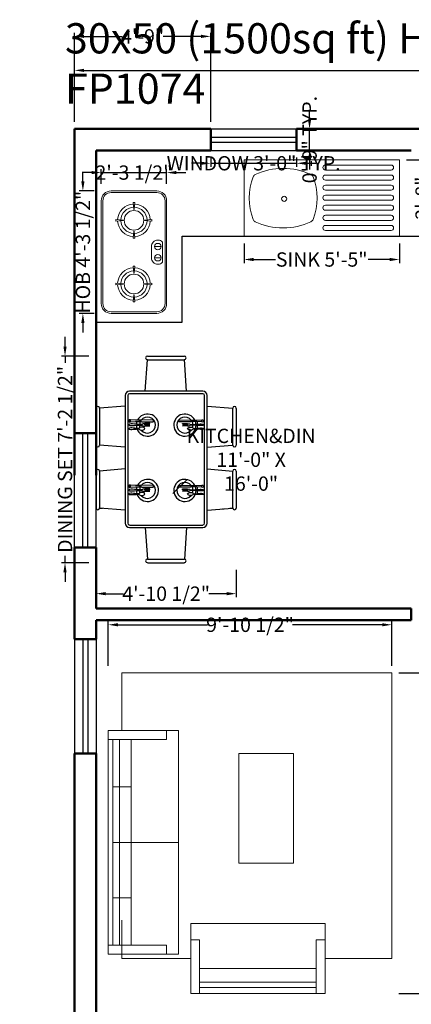
# Model space of a CAD drawing. Units: inches. Extents: x 234 to 707, y 260 to 1025.
# Tile 2 of 3: x 234 to 398, y 612 to 1025. Entities that reach past the tile are written whole.
import ezdxf

# ---------------------------------------------------------------- set-up
doc = ezdxf.new("R2010")
doc.units = ezdxf.units.IN
doc.header["$MEASUREMENT"] = 0
doc.layers.add('a patt', color=33, linetype='Continuous')
for name, color, linetype, lineweight in [('A-ANNO-DIMS', 3, 'Continuous', 18), ('A-ANNO-TEXT', 7, 'Continuous', 35), ('A-AREA-IDEN', 7, 'Continuous', 25), ('A-EQPM', 8, 'Continuous', 18), ('A-FLOR-CASE', 30, 'Continuous', 25), ('A-FLOR-FIXT', 9, 'Continuous', 18), ('A-FURN', 9, 'Continuous', 18), ('WALL', 7, 'Continuous', 50), ('WINDOW', 2, 'Continuous', 25)]:
    doc.layers.add(name, color=color, linetype=linetype, lineweight=lineweight)
doc.styles.get("Standard").update_dxf_attribs({"font": 'arial.ttf'})
doc.styles.add('YQ_DIM', font='SUPEROS.SHX', dxfattribs={"width": 0.8, "bigfont": 'HZDX.SHX'})
doc.dimstyles.new('yqi0', dxfattribs={"dimscale": 0, "dimtxt": 6, "dimasz": 4, "dimexe": 1.5, "dimexo": 3, "dimgap": 0.5, "dimtad": 0, "dimdec": 1, "dimdsep": 46, "dimlunit": 4, "dimtxsty": 'Standard', "dimcen": 0, "dimclrd": 256, "dimclre": 256, "dimclrt": 7, "dimadec": 1, "dimazin": 2, "dimtfac": 1, "dimtdec": 1, "dimtix": 1, "dimtmove": 2, "dimatfit": 2, "dimfxl": 1, "dimtolj": 1, "dimtzin": 0, "dimarcsym": 0})

# ---------------------------------------------------------------- blocks, each defined once
blk = doc.blocks.new('*D2')
at = {"layer": 'A-ANNO-DIMS', "color": 0, "lineweight": -2, "transparency": 16777216}
for p, q in [((257.21, 981.74), (257.21, 1004.79)), ((261.21, 1003.29), (431.62, 1003.29)), ((613.21, 1003.29), (442.8, 1003.29)), ((617.21, 981.74), (617.21, 1004.79))]:
    blk.add_line(p, q, dxfattribs=at)
at = {"layer": 'A-ANNO-DIMS', "color": 0, "transparency": 16777216}
for points in [[(261.21, 1003.95), (261.21, 1002.62), (257.21, 1003.29)], [(613.21, 1003.95), (613.21, 1002.62), (617.21, 1003.29)]]:
    blk.add_solid(points, dxfattribs=at)
at = {"layer": 'Defpoints', "color": 0, "transparency": 16777216}
for p in [(617.21, 1003.29), (257.21, 978.74), (617.21, 978.74)]:
    blk.add_point(p, dxfattribs=at)
at = {"layer": 'A-ANNO-DIMS', "color": 0, "transparency": 16777216, "insert": (437.21, 1003.29), "char_height": 6, "attachment_point": 5}
blk.add_mtext("\\A1;30'", dxfattribs=at)
blk = doc.blocks.new('WD_WIN4')
for p, q in [((-0.5, 0.5), (0.5, 0.5)), ((-0.5, 0.12), (0.5, 0.12)), ((-0.5, -0.12), (0.5, -0.12)), ((-0.5, -0.5), (0.5, -0.5))]:
    blk.add_line(p, q)
blk = doc.blocks.new('yq_cooker_01')
for p, q in [((426.3, 34.3), (465.5, 34.3)), ((426.3, -34.3), (465.5, -34.3))]:
    blk.add_line(p, q)
for points in [[(440, -375), (160, -375, -0.414214), (100, -315), (100, 315, -0.414214), (160, 375), (440, 375, -0.414214), (500, 315), (500, -315, -0.414214)], [(440, -365), (160, -365, -0.414214), (110, -315), (110, 315, -0.414214), (160, 365), (440, 365, -0.414214), (490, 315), (490, -315, -0.414214)]]:
    blk.add_lwpolyline(points, format="xyb", close=True)
for points in [[(300.8, 261.3), (305.4, 305), (294.6, 305), (299.2, 261.3)], [(233.7, 195.8), (190, 200.4), (190, 189.6), (233.7, 194.2)], [(366.3, 194.2), (410, 189.6), (410, 200.4), (366.3, 195.8)], [(299.2, 128.7), (294.6, 85), (305.4, 85), (300.8, 128.7)], [(299.2, -128.7), (294.6, -85), (305.4, -85), (300.8, -128.7)], [(233.7, -195.8), (190, -200.4), (190, -189.6), (233.7, -194.2)], [(366.3, -194.2), (410, -189.6), (410, -200.4), (366.3, -195.8)], [(300.8, -261.3), (305.4, -305), (294.6, -305), (299.2, -261.3)]]:
    blk.add_lwpolyline(points, close=True)
blk.add_lwpolyline([(406.7, -34.3, 0.414214), (445.9, -73.5), (455.5, -73.5, 0.414214), (475.1, -53.9), (475.1, 53.9, 0.414214), (455.5, 73.5), (445.9, 73.5, 0.414214), (406.7, 34.3), (406.7, -34.3)], format="xyb")
for centre, radius in [((300, 195), 60), ((445.9, 34.3), 19.6), ((445.9, -34.3), 19.6), ((300, -195), 60)]:
    blk.add_circle(centre, radius)
for centre, radius, start, end in [((300, 195), 100, 92.4978, 177.5022), ((300, 195), 80, 91.59131, 178.40869), ((300, 195), 80, 1.59131, 88.40869), ((300, 195), 100, 2.4978, 87.5022), ((300, 195), 100, 182.4978, 267.5022), ((300, 195), 80, 181.59131, 268.40869), ((300, 195), 80, 271.59131, 358.40869), ((300, 195), 100, 272.4978, 357.5022), ((300, -195), 100, 92.4978, 177.5022), ((300, -195), 80, 91.59131, 178.40869), ((300, -195), 80, 1.59131, 88.40869), ((300, -195), 100, 2.4978, 87.5022), ((300, -195), 100, 182.4978, 267.5022), ((300, -195), 80, 181.59131, 268.40869), ((300, -195), 80, 271.59131, 358.40869), ((300, -195), 100, 272.4978, 357.5022)]:
    blk.add_arc(centre, radius, start, end)
blk = doc.blocks.new('sink7a')
for p, q in [((12297, -765), (22250, -765)), ((12297, -1527), (22250, -1527)), ((12297, -2289), (22250, -2289)), ((12297, -3051), (22250, -3051)), ((12297, -3813), (22250, -3813)), ((12297, -4575), (22250, -4575)), ((12297, -5337), (22250, -5337)), ((12297, -6099), (22250, -6099)), ((12297, -6861), (22250, -6861)), ((12297, -7623), (22250, -7623)), ((12297, -8385), (22250, -8385)), ((12297, -9147), (22250, -9147)), ((12297, -9909), (22250, -9909)), ((12297, -10671), (22250, -10671))]:
    blk.add_line(p, q)
blk.add_lwpolyline([(0, 0), (0, -11557), (23495, -11557), (23495, 0)], close=True)
blk.add_lwpolyline([(1692, -9356, -0.193356), (1368, -9011, -0.1886606), (1376, -2541, -0.1929606), (1700, -2197, -0.2205414), (10111, -2197, -0.1929606), (10435, -2541, -0.1886606), (10443, -9011, -0.193356), (10119, -9356, -0.2209789)], format="xyb", close=True)
blk.add_circle((6064, -5888), 381)
for centre, start, end in [((12297, -1146), 90, 270), ((22250, -1146), 270, 90), ((12297, -2670), 90, 270), ((22250, -2670), 270, 90), ((12297, -4194), 90, 270), ((22250, -4194), 270, 90), ((12297, -5718), 90, 270), ((22250, -5718), 270, 90), ((12297, -7242), 90, 270), ((22250, -7242), 270, 90), ((12297, -8766), 90, 270), ((22250, -8766), 270, 90), ((12297, -10290), 90, 270), ((22250, -10290), 270, 90)]:
    blk.add_arc(centre, 381, start, end)
blk = doc.blocks.new('SOFA 21')
for p, q in [((-49.09, -24.34), (-49.09, 0)), ((37.16, -24.34), (37.16, 0)), ((-29.27, -1.86), (-49.09, -1.86)), ((-29.27, -9.53), (-29.27, -1.86)), ((-29.27, -1.86), (-5.97, -1.86)), ((17.33, -1.86), (-5.97, -1.86)), ((-5.97, -1.86), (-5.97, -9.53)), ((17.33, -9.53), (17.33, -1.86)), ((17.33, -1.86), (37.16, -1.86)), ((37.16, -4.72), (-49.09, -4.72)), ((37.16, -9.53), (-49.09, -9.53)), ((-5.97, -9.53), (-5.97, -29.38)), ((-52.84, -24.34), (-49.09, -24.34)), ((40.91, -24.34), (37.16, -24.34)), ((-46.78, -38.24), (-46.78, -34.49)), ((-46.78, -38.24), (-69.34, -38.24)), ((-66.74, -38.24), (-66.74, -86.99)), ((-64.62, -86.99), (-64.62, -38.24)), ((-58.88, -38.24), (-58.88, -86.99)), ((-46.78, -86.99), (-69.34, -86.99)), ((-46.78, -86.99), (-46.78, -90.74))]:
    blk.add_line(p, q)
for points in [[(40.91, -29.38), (-52.84, -29.38), (-52.84, 0), (40.91, 0)], [(-69.34, -34.49), (-69.34, -90.74), (-39.97, -90.74), (-39.97, -34.49)]]:
    blk.add_lwpolyline(points, close=True)
at = {"color": 0, "linetype": 'ByBlock', "lineweight": -2}
for points in [[(-54.65, -34.49), (-54.65, -5.62)], [(-54.65, -5.62), (-38.57, -5.62)], [(40.91, -5.62), (65.11, -5.62), (65.11, -118.7), (34.12, -118.7)], [(34.12, -118.7), (-54.65, -118.7), (-54.65, -90.74)]]:
    blk.add_lwpolyline(points, dxfattribs=at)
blk.add_lwpolyline([(-14.65, -77.55), (31.25, -77.55), (31.25, -54.6), (-14.65, -54.6)], close=True, dxfattribs=at)
blk = doc.blocks.new('grdfg')
at = {"layer": 'a patt'}
for p, q in [((589, 1028), (612, 1310)), ((609, 1310), (609, 1278)), ((615, 1349), (612, 1349)), ((1019, 1310), (612, 1310)), ((1016, 1349), (615, 1349)), ((615, 1349), (615, 1349)), ((1016, 1349), (1019, 1349)), ((1042, 1028), (1019, 1310)), ((1281, 1028), (1304, 1310)), ((1307, 1349), (1304, 1349)), ((1711, 1310), (1304, 1310)), ((1307, 1349), (1307, 1349)), ((1708, 1349), (1307, 1349)), ((1708, 1349), (1711, 1349)), ((1734, 1028), (1711, 1310)), ((605, 1201), (603, 1201)), ((1297, 1201), (1295, 1201)), ((397, 982), (397, 175)), ((425, 982), (425, 175)), ((1851, 1028), (444, 1028)), ((1851, 1000), (444, 1000)), ((1869, 175), (1869, 982)), ((1897, 175), (1897, 982)), ((763, 888), (769, 888)), ((763, 879), (769, 879)), ((841, 970), (863, 970)), ((845, 870), (859, 870)), ((1482, 888), (1488, 888)), ((1482, 879), (1488, 879)), ((1560, 970), (1582, 970)), ((1564, 870), (1578, 870)), ((10, 785), (10, 378)), ((397, 808), (49, 782)), ((49, 782), (49, 785)), ((49, 782), (49, 381)), ((813, 857), (806, 857)), ((806, 845), (813, 845)), ((845, 859), (859, 859)), ((845, 852), (859, 852)), ((1532, 857), (1525, 857)), ((1525, 845), (1532, 845)), ((1564, 859), (1578, 859)), ((1564, 852), (1578, 852)), ((1897, 808), (2245, 782)), ((2245, 782), (2246, 785)), ((2245, 782), (2245, 381)), ((2285, 785), (2285, 378)), ((770, 505), (923, 352)), ((49, 381), (49, 378)), ((49, 381), (49, 381)), ((397, 355), (49, 375)), ((1897, 355), (2246, 375)), ((2246, 381), (2245, 381)), ((2245, 381), (2246, 378)), ((763, 277), (769, 277)), ((763, 268), (769, 268)), ((771, 235), (802, 235)), ((806, 312), (813, 312)), ((813, 299), (806, 299)), ((816, 235), (844, 235)), ((845, 305), (859, 305)), ((845, 297), (859, 297)), ((845, 287), (859, 287)), ((1482, 277), (1488, 277)), ((1482, 268), (1488, 268)), ((1490, 235), (1521, 235)), ((1525, 312), (1532, 312)), ((1532, 299), (1525, 299)), ((1535, 235), (1563, 235)), ((1564, 305), (1578, 305)), ((1564, 297), (1578, 297)), ((1564, 287), (1578, 287)), ((444, 156), (1851, 156)), ((444, 128), (1851, 128)), ((589, 128), (612, -153)), ((841, 187), (863, 187)), ((1042, 128), (1019, -154)), ((1281, 128), (1304, -153)), ((1560, 187), (1582, 187)), ((1734, 128), (1711, -154)), ((605, -45), (603, -45)), ((1028, -45), (1026, -45)), ((609, -122), (609, -154)), ((1019, -153), (612, -153)), ((615, -193), (612, -193)), ((615, -192), (615, -193)), ((1016, -193), (615, -193)), ((1016, -193), (1019, -193)), ((1711, -153), (1304, -153)), ((1307, -193), (1304, -193)), ((1307, -192), (1307, -193)), ((1708, -193), (1307, -193)), ((1708, -193), (1711, -193))]:
    blk.add_line(p, q, dxfattribs=at)
for points in [[(759, 967), (759, 955, -0.013852), (763, 888), (763, 879, -0.321801), (758, 871, 0.220637), (749, 856, 0.151079), (756, 820, 0.601255), (777, 820, 0.098298), (784, 846, 0.173345), (779, 867, 0.127575), (772, 873, -0.108886), (769, 879), (769, 888, -0.013852), (774, 955), (774, 967), (772, 982, 0.903848), (760, 982)], [(841, 986, 0.204141), (841, 970), (845, 914), (845, 870), (843, 863), (845, 859), (845, 852), (843, 847, -0.015744), (841, 722, 0.538165), (859, 722), (864, 847), (859, 852), (859, 859), (861, 863), (859, 870), (859, 914), (863, 970, 0.204141), (863, 986), (857, 988), (847, 988)], [(1478, 967), (1478, 955, -0.013852), (1482, 888), (1482, 879, -0.321801), (1477, 871, 0.220637), (1468, 856, 0.151079), (1475, 820, 0.601255), (1496, 820, 0.098298), (1503, 846, 0.173345), (1498, 867, 0.127575), (1491, 873, -0.108886), (1488, 879), (1488, 888, -0.013852), (1493, 955), (1493, 967), (1491, 982, 0.903848), (1479, 982)], [(1560, 986, 0.204141), (1560, 970), (1564, 914), (1564, 870), (1562, 863), (1564, 859), (1564, 852), (1562, 847, -0.015744), (1560, 722, 0.538165), (1578, 722), (1583, 847), (1578, 852), (1578, 859), (1580, 863), (1578, 870), (1578, 914), (1582, 970, 0.204141), (1582, 986), (1576, 988), (1566, 988)], [(841, 171, -0.204141), (841, 187), (845, 242), (845, 287), (843, 294), (845, 297), (845, 305), (843, 310, 0.015744), (841, 435, -0.538165), (859, 435), (864, 310), (859, 305), (859, 297), (861, 294), (859, 287), (859, 242), (863, 187, -0.204141), (863, 171), (857, 169), (847, 169)], [(1560, 171, -0.204141), (1560, 187), (1564, 242), (1564, 287), (1562, 294), (1564, 297), (1564, 305), (1562, 310, 0.015744), (1560, 435, -0.538165), (1578, 435), (1583, 310), (1578, 305), (1578, 297), (1580, 294), (1578, 287), (1578, 242), (1582, 187, -0.204141), (1582, 171), (1576, 169), (1566, 169)], [(759, 189), (759, 202, 0.013852), (763, 268), (763, 277, 0.321801), (758, 285, -0.220637), (749, 300, -0.151079), (756, 336, -0.601255), (777, 336, -0.098298), (784, 311, -0.173345), (779, 289, -0.127575), (772, 283, 0.108886), (769, 277), (769, 268, 0.013852), (774, 202), (774, 189), (772, 174, -0.903848), (760, 174)], [(1478, 189), (1478, 202, 0.013852), (1482, 268), (1482, 277, 0.321801), (1477, 285, -0.220637), (1468, 300, -0.151079), (1475, 336, -0.601255), (1496, 336, -0.098298), (1503, 311, -0.173345), (1498, 289, -0.127575), (1491, 283, 0.108886), (1488, 277), (1488, 268, 0.013852), (1493, 202), (1493, 189), (1491, 174, -0.903848), (1479, 174)]]:
    blk.add_lwpolyline(points, format="xyb", close=True, dxfattribs=at)
for points in [[(802, 982), (800, 964), (800, 950, -0.012883), (806, 857), (806, 845, -0.236068), (798, 834, 0.098033), (795, 814), (797, 759), (798, 759), (800, 814), (802, 814), (804, 759), (806, 759), (807, 816), (809, 818), (811, 816), (813, 759), (814, 759), (816, 814), (818, 814), (820, 759), (822, 759), (823, 814), (820, 834, -0.236068), (813, 845), (813, 857, -0.012883), (818, 950), (818, 964), (816, 982, 0.761905), (802, 982, 0.027392)], [(1521, 982), (1519, 964), (1519, 950, -0.012883), (1525, 857), (1525, 845, -0.236068), (1517, 834, 0.098033), (1514, 814), (1516, 759), (1517, 759), (1519, 814), (1521, 814), (1523, 759), (1525, 759), (1526, 816), (1528, 818), (1530, 816), (1532, 759), (1533, 759), (1535, 814), (1537, 814), (1539, 759), (1541, 759), (1542, 814), (1539, 834, -0.236068), (1532, 845), (1532, 857, -0.012883), (1537, 950), (1537, 964), (1535, 982, 0.761905), (1521, 982, 0.027392)], [(802, 174), (800, 192), (800, 206, 0.012883), (806, 299), (806, 312, 0.236068), (798, 322, -0.098033), (795, 342), (797, 397), (798, 397), (800, 342), (802, 342), (804, 397), (806, 397), (807, 340), (809, 338), (811, 340), (813, 397), (814, 397), (816, 342), (818, 342), (820, 397), (822, 397), (823, 342), (820, 322, 0.236068), (813, 312), (813, 299, 0.012883), (818, 206), (818, 192), (816, 174, -0.761905), (802, 174, -0.027392)], [(1521, 174), (1519, 192), (1519, 206, 0.012883), (1525, 299), (1525, 312, 0.236068), (1517, 322, -0.098033), (1514, 342), (1516, 397), (1517, 397), (1519, 342), (1521, 342), (1523, 397), (1525, 397), (1526, 340), (1528, 338), (1530, 340), (1532, 397), (1533, 397), (1535, 342), (1537, 342), (1539, 397), (1541, 397), (1542, 342), (1539, 322, 0.236068), (1532, 312), (1532, 299, 0.012883), (1537, 206), (1537, 192), (1535, 174, -0.761905), (1521, 174, -0.027392)]]:
    blk.add_lwpolyline(points, format="xyb", dxfattribs=at)
for centre, radius, start, end in [((613, 1329), 19.5, 92.4912, 267.9051), ((1018, 1329), 19.5, 272.0949, 87.5088), ((1305, 1329), 19.5, 92.4912, 267.9051), ((1710, 1329), 19.5, 272.0949, 87.5088), ((444, 982), 46.6, 90, 180), ((444, 982), 18.7, 90, 180), ((1851, 982), 46.6, 0, 90), ((1851, 982), 18.7, 0, 90), ((806, 784), 122, 110.569, 64.0676), ((806, 784), 122, 91.1026, 107.1168), ((806, 784), 88.4, 90.4281, 108.0635), ((806, 784), 88.4, 64.8376, 85.191), ((806, 784), 122, 71.3681, 85.7295), ((1525, 784), 122, 110.569, 64.0676), ((1525, 784), 122, 91.1026, 107.1168), ((1525, 784), 88.4, 90.4281, 108.0635), ((1525, 784), 88.4, 64.8376, 85.191), ((1525, 784), 122, 71.3681, 85.7295), ((30, 784), 19.5, 2.4912, 177.9051), ((806, 784), 88.4, 130.4177, 52.8326), ((1525, 784), 88.4, 130.4177, 52.8326), ((2265, 784), 19.5, 2.0949, 177.5088), ((806, 372), 122, 295.9324, 249.431), ((806, 372), 88.4, 307.1674, 229.5823), ((1525, 372), 122, 295.9324, 249.431), ((1525, 372), 88.4, 307.1674, 229.5823), ((30, 379), 19.5, 182.0949, 357.5088), ((2265, 379), 19.5, 182.4912, 357.9051), ((806, 372), 122, 252.8832, 268.8974), ((806, 372), 88.4, 251.9365, 269.5719), ((806, 372), 88.4, 274.809, 295.1624), ((806, 372), 122, 274.2705, 288.6319), ((1525, 372), 122, 252.8832, 268.8974), ((1525, 372), 88.4, 251.9365, 269.5719), ((1525, 372), 88.4, 274.809, 295.1624), ((1525, 372), 122, 274.2705, 288.6319), ((444, 175), 46.6, 180, 270), ((444, 175), 18.7, 180, 270), ((1851, 175), 46.6, 270, 0), ((1851, 175), 18.7, 270, 0), ((613, -173), 19.5, 92.0949, 267.5088), ((1018, -173), 19.5, 272.4912, 87.9051), ((1305, -173), 19.5, 92.0949, 267.5088), ((1710, -173), 19.5, 272.4912, 87.9051)]:
    blk.add_arc(centre, radius, start, end, dxfattribs=at)
blk = doc.blocks.new('*D23')
at = {"layer": 'A-ANNO-DIMS', "lineweight": -2, "transparency": 16777216}
for p, q in [((314.21, 966.74), (314.21, 962.84)), ((350.21, 966.74), (350.21, 962.84)), ((310.21, 964.34), (306.21, 964.34)), ((314.21, 964.34), (350.21, 964.34)), ((354.21, 964.34), (358.21, 964.34))]:
    blk.add_line(p, q, dxfattribs=at)
at = {"layer": 'A-ANNO-DIMS', "transparency": 16777216}
for points in [[(310.21, 965.01), (310.21, 963.67), (314.21, 964.34)], [(354.21, 965.01), (354.21, 963.67), (350.21, 964.34)]]:
    blk.add_solid(points, dxfattribs=at)
at = {"layer": 'Defpoints', "color": 0, "transparency": 16777216}
for p in [(314.21, 969.74), (350.21, 969.74), (350.21, 964.34)]:
    blk.add_point(p, dxfattribs=at)
at = {"layer": 'A-ANNO-DIMS', "color": 7, "transparency": 16777216, "insert": (332.21, 964.34), "char_height": 6, "attachment_point": 5}
blk.add_mtext('\\A1;WINDOW 3\'-0" TYP.', dxfattribs=at)
blk = doc.blocks.new('*D24')
at = {"layer": 'A-ANNO-DIMS', "lineweight": -2, "transparency": 16777216}
for p, q in [((355.61, 982.74), (355.61, 986.74)), ((353.21, 978.74), (357.11, 978.74)), ((355.61, 969.74), (355.61, 978.74)), ((353.21, 969.74), (357.11, 969.74)), ((355.61, 965.74), (355.61, 961.74))]:
    blk.add_line(p, q, dxfattribs=at)
at = {"layer": 'A-ANNO-DIMS', "transparency": 16777216}
for points in [[(354.95, 982.74), (356.28, 982.74), (355.61, 978.74)], [(354.95, 965.74), (356.28, 965.74), (355.61, 969.74)]]:
    blk.add_solid(points, dxfattribs=at)
at = {"layer": 'Defpoints', "color": 0, "transparency": 16777216}
for p in [(350.21, 978.74), (355.61, 978.74), (350.21, 969.74)]:
    blk.add_point(p, dxfattribs=at)
at = {"layer": 'A-ANNO-DIMS', "color": 7, "transparency": 16777216, "insert": (355.61, 974.24), "char_height": 6, "attachment_point": 5, "rotation": 90}
blk.add_mtext('\\A1;0\'-9" TYP.', dxfattribs=at)
blk = doc.blocks.new('*D39')
at = {"layer": 'A-ANNO-DIMS', "lineweight": -2, "transparency": 16777216}
for p, q in [((260.71, 956.73), (260.71, 960.73)), ((265.41, 952.73), (259.21, 952.73)), ((260.71, 952.73), (260.71, 952.62)), ((265.41, 901.4), (259.21, 901.4)), ((260.71, 901.4), (260.71, 901.52)), ((260.71, 897.4), (260.71, 893.4))]:
    blk.add_line(p, q, dxfattribs=at)
at = {"layer": 'A-ANNO-DIMS', "transparency": 16777216}
for points in [[(260.04, 956.73), (261.37, 956.73), (260.71, 952.73)], [(260.04, 897.4), (261.37, 897.4), (260.71, 901.4)]]:
    blk.add_solid(points, dxfattribs=at)
at = {"layer": 'Defpoints', "color": 0, "transparency": 16777216}
for p in [(260.71, 952.73), (268.41, 952.73), (268.41, 901.4)]:
    blk.add_point(p, dxfattribs=at)
at = {"layer": 'A-ANNO-DIMS', "color": 7, "transparency": 16777216, "insert": (260.71, 927.07), "char_height": 6, "attachment_point": 5, "rotation": 90}
blk.add_mtext('\\A1;HOB 4\'-3 1/2"', dxfattribs=at)
blk = doc.blocks.new('*D40')
at = {"layer": 'A-ANNO-DIMS', "lineweight": -2, "transparency": 16777216}
for p, q in [((268.41, 955.73), (268.41, 961.93)), ((295.78, 955.73), (295.78, 961.93)), ((264.41, 960.43), (260.41, 960.43)), ((268.41, 960.43), (295.78, 960.43)), ((299.78, 960.43), (303.78, 960.43))]:
    blk.add_line(p, q, dxfattribs=at)
at = {"layer": 'A-ANNO-DIMS', "transparency": 16777216}
for points in [[(264.41, 961.1), (264.41, 959.77), (268.41, 960.43)], [(299.78, 961.1), (299.78, 959.77), (295.78, 960.43)]]:
    blk.add_solid(points, dxfattribs=at)
at = {"layer": 'Defpoints', "color": 0, "transparency": 16777216}
for p in [(295.78, 960.43), (268.41, 952.73), (295.78, 952.73)]:
    blk.add_point(p, dxfattribs=at)
at = {"layer": 'A-ANNO-DIMS', "color": 7, "transparency": 16777216, "insert": (282.09, 960.43), "char_height": 6, "attachment_point": 5}
blk.add_mtext('\\A1;2\'-3 1/2"', dxfattribs=at)
blk = doc.blocks.new('*D41')
at = {"layer": 'A-ANNO-DIMS', "lineweight": -2, "transparency": 16777216}
for p, q in [((328.2, 930.74), (328.2, 922.49)), ((393.21, 930.74), (393.21, 922.49)), ((332.2, 923.99), (341.3, 923.99)), ((389.21, 923.99), (380.11, 923.99))]:
    blk.add_line(p, q, dxfattribs=at)
at = {"layer": 'A-ANNO-DIMS', "transparency": 16777216}
for points in [[(332.2, 924.66), (332.2, 923.32), (328.2, 923.99)], [(389.21, 924.66), (389.21, 923.32), (393.21, 923.99)]]:
    blk.add_solid(points, dxfattribs=at)
at = {"layer": 'Defpoints', "color": 0, "transparency": 16777216}
for p in [(328.2, 933.74), (393.21, 933.74), (393.21, 923.99)]:
    blk.add_point(p, dxfattribs=at)
at = {"layer": 'A-ANNO-DIMS', "color": 7, "transparency": 16777216, "insert": (360.7, 923.99), "char_height": 6, "attachment_point": 5}
blk.add_mtext('\\A1;SINK 5\'-5"', dxfattribs=at)
blk = doc.blocks.new('*D42')
at = {"layer": 'A-ANNO-DIMS', "lineweight": -2, "transparency": 16777216}
for p, q in [((396.21, 965.72), (404.46, 965.72)), ((402.96, 961.72), (402.96, 958.26)), ((402.96, 937.74), (402.96, 941.21)), ((396.21, 933.74), (404.46, 933.74))]:
    blk.add_line(p, q, dxfattribs=at)
at = {"layer": 'A-ANNO-DIMS', "transparency": 16777216}
for points in [[(402.3, 961.72), (403.63, 961.72), (402.96, 965.72)], [(402.3, 937.74), (403.63, 937.74), (402.96, 933.74)]]:
    blk.add_solid(points, dxfattribs=at)
at = {"layer": 'Defpoints', "color": 0, "transparency": 16777216}
for p in [(393.21, 965.72), (402.96, 965.72), (393.21, 933.74)]:
    blk.add_point(p, dxfattribs=at)
at = {"layer": 'A-ANNO-DIMS', "color": 7, "transparency": 16777216, "insert": (402.96, 949.73), "char_height": 6, "attachment_point": 5, "rotation": 90}
blk.add_mtext('\\A1;2\'-8"', dxfattribs=at)
blk = doc.blocks.new('*D45')
at = {"layer": 'A-ANNO-DIMS', "lineweight": -2, "transparency": 16777216}
for p, q in [((393.05, 750.69), (411.72, 750.69)), ((410.22, 746.69), (410.22, 729.31)), ((410.22, 620.24), (410.22, 637.63)), ((393.05, 616.24), (411.72, 616.24))]:
    blk.add_line(p, q, dxfattribs=at)
at = {"layer": 'A-ANNO-DIMS', "transparency": 16777216}
for points in [[(409.55, 746.69), (410.88, 746.69), (410.22, 750.69)], [(409.55, 620.24), (410.88, 620.24), (410.22, 616.24)]]:
    blk.add_solid(points, dxfattribs=at)
at = {"layer": 'Defpoints', "color": 0, "transparency": 16777216}
for p in [(390.05, 750.69), (410.22, 750.69), (390.05, 616.24)]:
    blk.add_point(p, dxfattribs=at)
at = {"layer": 'A-ANNO-DIMS', "color": 7, "transparency": 16777216, "insert": (410.22, 683.47), "char_height": 6, "attachment_point": 5, "rotation": 90}
blk.add_mtext('\\A1;LOUNGE SET 11\'-2 1/2"', dxfattribs=at)
blk = doc.blocks.new('*D46')
at = {"layer": 'A-ANNO-DIMS', "lineweight": -2, "transparency": 16777216}
for p, q in [((271.35, 753.69), (271.35, 772.36)), ((390.05, 753.69), (390.05, 772.36)), ((275.35, 770.86), (312.9, 770.86)), ((386.05, 770.86), (348.49, 770.86))]:
    blk.add_line(p, q, dxfattribs=at)
at = {"layer": 'A-ANNO-DIMS', "transparency": 16777216}
for points in [[(275.35, 771.52), (275.35, 770.19), (271.35, 770.86)], [(386.05, 771.52), (386.05, 770.19), (390.05, 770.86)]]:
    blk.add_solid(points, dxfattribs=at)
at = {"layer": 'Defpoints', "color": 0, "transparency": 16777216}
for p in [(271.35, 770.86), (271.35, 750.69), (390.05, 750.69)]:
    blk.add_point(p, dxfattribs=at)
at = {"layer": 'A-ANNO-DIMS', "color": 7, "transparency": 16777216, "insert": (330.7, 770.86), "char_height": 6, "attachment_point": 5}
blk.add_mtext('\\A1;9\'-10 1/2"', dxfattribs=at)
blk = doc.blocks.new('*D47')
at = {"layer": 'A-ANNO-DIMS', "lineweight": -2, "transparency": 16777216}
for p, q in [((253.22, 887.51), (253.22, 891.51)), ((263.21, 883.51), (251.72, 883.51)), ((253.22, 883.51), (253.22, 880.66)), ((263.21, 796.88), (251.72, 796.88)), ((253.22, 796.88), (253.22, 799.73)), ((253.22, 792.88), (253.22, 788.88))]:
    blk.add_line(p, q, dxfattribs=at)
at = {"layer": 'A-ANNO-DIMS', "transparency": 16777216}
for points in [[(252.55, 887.51), (253.89, 887.51), (253.22, 883.51)], [(252.55, 792.88), (253.89, 792.88), (253.22, 796.88)]]:
    blk.add_solid(points, dxfattribs=at)
at = {"layer": 'Defpoints', "color": 0, "transparency": 16777216}
for p in [(253.22, 883.51), (266.21, 883.51), (266.21, 796.88)]:
    blk.add_point(p, dxfattribs=at)
at = {"layer": 'A-ANNO-DIMS', "color": 7, "transparency": 16777216, "insert": (253.22, 840.2), "char_height": 6, "attachment_point": 5, "rotation": 90}
blk.add_mtext('\\A1;DINING SET 7\'-2 1/2"', dxfattribs=at)
blk = doc.blocks.new('*D48')
at = {"layer": 'A-ANNO-DIMS', "lineweight": -2, "transparency": 16777216}
for p, q in [((266.21, 793.88), (266.21, 782.39)), ((324.93, 793.88), (324.93, 782.39)), ((270.21, 783.89), (277.65, 783.89)), ((320.93, 783.89), (313.49, 783.89))]:
    blk.add_line(p, q, dxfattribs=at)
at = {"layer": 'A-ANNO-DIMS', "transparency": 16777216}
for points in [[(270.21, 784.56), (270.21, 783.22), (266.21, 783.89)], [(320.93, 784.56), (320.93, 783.22), (324.93, 783.89)]]:
    blk.add_solid(points, dxfattribs=at)
at = {"layer": 'Defpoints', "color": 0, "transparency": 16777216}
for p in [(266.21, 796.88), (324.93, 796.88), (266.21, 783.89)]:
    blk.add_point(p, dxfattribs=at)
at = {"layer": 'A-ANNO-DIMS', "color": 7, "transparency": 16777216, "insert": (295.57, 783.89), "char_height": 6, "attachment_point": 5}
blk.add_mtext('\\A1;4\'-10 1/2"', dxfattribs=at)
blk = doc.blocks.new('*D51')
at = {"layer": 'A-ANNO-DIMS', "lineweight": -2, "transparency": 16777216}
for p, q in [((257.21, 981.74), (257.21, 1019.04)), ((261.21, 1017.54), (277.12, 1017.54)), ((310.21, 1017.54), (294.31, 1017.54)), ((314.21, 981.74), (314.21, 1019.04))]:
    blk.add_line(p, q, dxfattribs=at)
at = {"layer": 'A-ANNO-DIMS', "transparency": 16777216}
for points in [[(261.21, 1018.21), (261.21, 1016.87), (257.21, 1017.54)], [(310.21, 1018.21), (310.21, 1016.87), (314.21, 1017.54)]]:
    blk.add_solid(points, dxfattribs=at)
at = {"layer": 'Defpoints', "color": 0, "transparency": 16777216}
for p in [(314.21, 1017.54), (257.21, 978.74), (314.21, 978.74)]:
    blk.add_point(p, dxfattribs=at)
at = {"layer": 'A-ANNO-DIMS', "color": 7, "transparency": 16777216, "insert": (285.71, 1017.54), "char_height": 6, "attachment_point": 5}
blk.add_mtext('\\A1;4\'-9"', dxfattribs=at)

msp = doc.modelspace()

# ---------------------------------------------------------------- linework, layer by layer
at = {"layer": 'A-FLOR-CASE'}
for p, q in [((302.21, 933.74), (398.21, 933.74)), ((302.21, 897.74), (302.21, 933.74)), ((266.21, 897.74), (302.21, 897.74))]:
    msp.add_line(p, q, dxfattribs=at)
at = {"layer": 'WALL'}
for p, q in [((257.21, 978.74), (314.21, 978.74)), ((257.21, 833.62), (257.21, 978.74)), ((314.21, 969.74), (314.21, 978.74)), ((350.21, 978.74), (425.21, 978.74)), ((350.21, 969.74), (350.21, 978.74)), ((266.21, 969.74), (314.21, 969.74)), ((266.21, 833.62), (266.21, 969.74)), ((350.21, 969.74), (398.21, 969.74)), ((266.21, 851.24), (257.21, 851.24)), ((266.21, 803.24), (257.21, 803.24)), ((257.21, 764.87), (257.21, 803.24)), ((266.21, 777.74), (266.21, 803.24)), ((266.21, 777.74), (398.21, 777.74)), ((398.21, 777.74), (398.21, 772.74)), ((266.21, 772.74), (398.21, 772.74)), ((266.21, 764.87), (266.21, 772.74)), ((266.21, 764.87), (257.21, 764.87)), ((266.21, 716.87), (257.21, 716.87)), ((257.21, 574.62), (257.21, 716.87)), ((266.21, 574.62), (266.21, 716.87))]:
    msp.add_line(p, q, dxfattribs=at)

# ---------------------------------------------------------------- block references
at = {"layer": 'A-EQPM', "xscale": 0.0684420978957593, "yscale": 0.0684420978957593, "zscale": 0.0684420978957593}
msp.add_blockref('yq_cooker_01', (261.56, 927.07), dxfattribs=at)
at = {"layer": 'A-FLOR-FIXT', "xscale": 0.0027671340803704, "yscale": 0.0027671340803704, "zscale": 0.0027671340803704}
msp.add_blockref('sink7a', (328.2, 965.72), dxfattribs=at)
at = {"layer": 'A-FURN', "xscale": 0.0380835584416279, "yscale": 0.0380835584416279, "zscale": 0.0380835584416279, "rotation": 90}
msp.add_blockref('grdfg', (317.59, 796.5), dxfattribs=at)
at = {"layer": 'A-FURN', "rotation": 89.99999999999999}
msp.add_blockref('SOFA 21', (271.35, 685.59), dxfattribs=at)
at = {"layer": 'WINDOW', "xscale": 36, "yscale": 9.000000000000455, "zscale": 36}
msp.add_blockref('WD_WIN4', (332.21, 974.24), dxfattribs=at)
at = {"layer": 'WINDOW', "xscale": 48, "zscale": 48}
for p, yscale, rotation in [((261.71, 827.24), 8.99999999999909, 89.99999999999973), ((261.71, 740.87), 8.999999999999261, 269.9999999999998)]:
    msp.add_blockref('WD_WIN4', p, dxfattribs=dict(at, yscale=yscale, rotation=rotation))

# ---------------------------------------------------------------- texts
at = {"layer": 'A-ANNO-TEXT', "insert": (253.19, 1023.06), "char_height": 12.6649, "width": 382.1676, "attachment_point": 1, "style": 'YQ_DIM'}
msp.add_mtext('30x50 (1500sq ft) House Plan - North face - FP1074', dxfattribs=at)
at = {"layer": 'A-AREA-IDEN', "insert": (305.99, 853.04), "char_height": 13.7795, "width": 50.2899, "attachment_point": 1, "style": 'YQ_DIM'}
msp.add_mtext('\\pxqc;{\\H0.43543x;KITCHEN&DIN\\P11\'-0" X 16\'-0"}', dxfattribs=at)

# ---------------------------------------------------------------- dimensions: what is measured, and where the dimension line sits
at = {"layer": 'A-ANNO-DIMS'}
for base, p1, p2, picture, middle in [((314.21, 1017.54), (257.21, 978.74), (314.21, 978.74), '*D51', (285.71, 1017.54)), ((295.78, 960.43), (268.41, 952.73), (295.78, 952.73), '*D40', (282.09, 960.43))]:
    dim = msp.add_linear_dim(base=base, p1=p1, p2=p2, dimstyle='yqi0', override={"dimscale": 1, "dimzin": 1, "dimfrac": 2}, dxfattribs=at)
    dim.commit()
    dim.dimension.update_dxf_attribs({"geometry": picture, "text_midpoint": middle})
dim = msp.add_aligned_dim(p1=(257.21, 978.74), p2=(617.21, 978.74), distance=24.55, dimstyle='yqi0', override={"dimscale": 1, "dimclrd": 0, "dimclre": 0, "dimclrt": 0}, dxfattribs=at)
dim.commit()
dim.dimension.update_dxf_attribs({"geometry": '*D2', "text_midpoint": (437.21, 1003.29)})
for base, p1, p2, text, picture, middle in [((355.61, 978.74), (350.21, 969.74), (350.21, 978.74), '<> TYP.', '*D24', (355.61, 974.24)), ((260.71, 952.73), (268.41, 901.4), (268.41, 952.73), 'HOB <>', '*D39', (260.71, 927.07)), ((253.22, 883.51), (266.21, 796.88), (266.21, 883.51), 'DINING SET <>', '*D47', (253.22, 840.2)), ((410.2171, 750.6913), (390.0501, 616.2445), (390.0501, 750.6913), 'LOUNGE SET <>', '*D45', (410.2171, 683.4679))]:
    dim = msp.add_linear_dim(base=base, p1=p1, p2=p2, angle=90, text=text, dimstyle='yqi0', override={"dimscale": 1, "dimzin": 1, "dimfrac": 2}, dxfattribs=at)
    dim.commit()
    dim.dimension.update_dxf_attribs({"geometry": picture, "text_midpoint": middle})
for base, p1, p2, text, picture, middle in [((350.21, 964.34), (314.21, 969.74), (350.21, 969.74), 'WINDOW <> TYP.', '*D23', (332.21, 964.34)), ((393.21, 923.99), (328.2, 933.74), (393.21, 933.74), 'SINK <>', '*D41', (360.7, 923.99))]:
    dim = msp.add_linear_dim(base=base, p1=p1, p2=p2, text=text, dimstyle='yqi0', override={"dimscale": 1, "dimzin": 1, "dimfrac": 2}, dxfattribs=at)
    dim.commit()
    dim.dimension.update_dxf_attribs({"geometry": picture, "text_midpoint": middle})
for base, p1, p2, angle, picture, middle in [((402.96, 965.72), (393.21, 933.74), (393.21, 965.72), 90, '*D42', (402.96, 949.73)), ((266.21, 783.89), (324.93, 796.88), (266.21, 796.88), 180, '*D48', (295.57, 783.89)), ((271.35, 770.86), (390.05, 750.69), (271.35, 750.69), 180, '*D46', (330.7, 770.86))]:
    dim = msp.add_linear_dim(base=base, p1=p1, p2=p2, angle=angle, dimstyle='yqi0', override={"dimscale": 1, "dimzin": 1, "dimfrac": 2}, dxfattribs=at)
    dim.commit()
    dim.dimension.update_dxf_attribs({"geometry": picture, "text_midpoint": middle})

doc.saveas('drawing.dxf')
